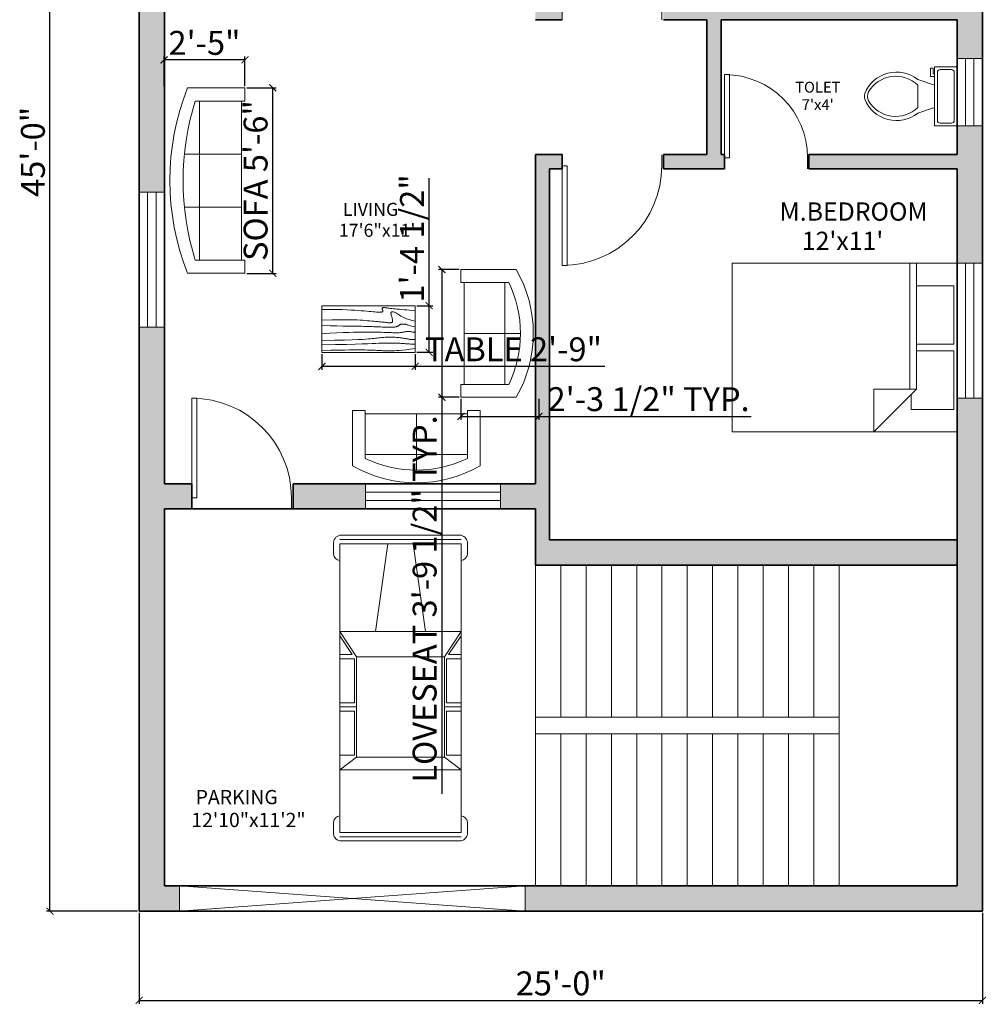
# Model space of a CAD drawing. Units: inches. Extents: x 3799 to 20199, y 1682 to 8087.
# Tile 26 of 30: x 16248 to 16592, y 7462 to 7812. Entities that reach past the tile are written whole.
import ezdxf

# ---------------------------------------------------------------- set-up
doc = ezdxf.new("R2010")
doc.units = ezdxf.units.IN
for name, color, linetype, lineweight in [('A-ANNO-DIMS', 2, 'Continuous', 18), ('A-AREA-IDEN', 7, 'Continuous', 18), ('A-DOOR', 3, 'Continuous', 18), ('A-FLOR-FIXT', 9, 'Continuous', 18), ('A-FLOR-STRS', 41, 'Continuous', 18), ('A-FURN', 8, 'Continuous', 18), ('A-GLAZ', 152, 'Continuous', 18), ('A-SITE-VEHC', 8, 'Continuous', 13), ('A-WALL', 7, 'Continuous', 35), ('A-WALL-PATT', 252, 'Continuous', 13)]:
    doc.layers.add(name, color=color, linetype=linetype, lineweight=lineweight)
doc.styles.get("Standard").update_dxf_attribs({"font": 'arial.ttf'})
doc.dimstyles.new('ISO-25', dxfattribs={"dimtxt": 8.5, "dimasz": 2.5, "dimexe": 1.25, "dimexo": 0.625, "dimtad": 1, "dimdec": 0, "dimlunit": 3, "dimtxsty": 'Standard', "dimblk": 'ARCHTICK', "dimcen": 2.5, "dimadec": 0, "dimazin": 0, "dimtfac": 1, "dimtdec": 0, "dimtmove": 0, "dimatfit": 3, "dimfxl": 1, "dimarcsym": 0})

# ---------------------------------------------------------------- blocks, each defined once
blk = doc.blocks.new('Sofa - Roundback Loveseat 5 ft.')
for p, q in [((0, -32.44198), (0, -5.99998)), ((-24, -33.99998), (-24, -11.46958)), ((-23.9998, -13.38178), (23.99986, -13.38178)), ((24.00004, -33.99998), (24.00004, -11.46958)), ((-24, -32.44198), (24.00004, -32.44198))]:
    blk.add_line(p, q)
for points in [[(-24, -33.99998), (-30, -33.99998), (-30, -7.99998)], [(30.00004, -7.99998), (30.00004, -33.99998), (24.00004, -33.99998)]]:
    blk.add_lwpolyline(points)
for centre, radius, start, end in [((0, -60.24998), 60.24998, 60.13715, 119.8628), ((0, -61.38438), 55.38444, 64.32083, 115.6792)]:
    blk.add_arc(centre, radius, start, end)
blk = doc.blocks.new('Sofa - Roundback 7 ft.')
for p, q in [((-12.00002, -32.4421), (-12.00003, -6.5971)), ((11.99997, -32.4421), (11.99998, -6.5971)), ((-36.000027, -34), (-36.000027, -11.4696)), ((35.99998, -34), (35.99998, -11.4696)), ((-35.999844, -13.3819), (35.9998, -13.3819)), ((-36.000027, -32.4421), (35.99998, -32.4421))]:
    blk.add_line(p, q)
for points in [[(-36.000027, -34), (-42.000027, -34), (-42.000027, -8)], [(41.99998, -8), (41.99998, -34), (35.99998, -34)]]:
    blk.add_lwpolyline(points)
for centre, radius, start, end in [((0, -114.25), 114.25, 68.43141, 111.5686), ((-0.00001, -127.1968), 121.1968, 72.72033, 107.2797)]:
    blk.add_arc(centre, radius, start, end)
blk = doc.blocks.new('Table - Rectangular Woodgrain 60 x 30 in.')
for p, q in [((0, 0), (0, -30)), ((60, 0), (0, 0)), ((60, -30), (60, 0)), ((0, -30), (60, -30))]:
    blk.add_line(p, q)
for points in [[(0, -2.4), (4.8155, -2.418), (9.0302, -2.4688), (12.709, -2.5477), (15.9167, -2.65), (18.7181, -2.7711), (21.1781, -2.9063), (23.3616, -3.0508), (25.3333, -3.2), (27.1477, -3.3495), (28.8172, -3.4958), (30.3437, -3.636), (31.7291, -3.7667), (32.9756, -3.8849), (34.0849, -3.9875), (35.059, -4.0714), (35.9, -4.1334), (36.6114, -4.1711), (37.2041, -4.1854), (37.6906, -4.1779), (38.0833, -4.15), (38.3948, -4.1034), (38.6375, -4.0396), (38.8239, -3.9602), (38.9666, -3.8667), (39.0764, -3.7608), (39.1573, -3.6448), (39.2116, -3.521), (39.2416, -3.3917), (39.2498, -3.2593), (39.2385, -3.1261), (39.21, -2.9944), (39.1666, -2.8667), (39.111, -2.7447), (39.0468, -2.6281), (38.978, -2.5163), (38.9083, -2.4083), (38.8418, -2.3035), (38.7823, -2.201), (38.7337, -2.1001), (38.7, -2), (38.6844, -1.9003), (38.6875, -1.8021), (38.7094, -1.707), (38.75, -1.6167), (38.8094, -1.5326), (38.8875, -1.4563), (38.9844, -1.3893), (39.1, -1.3333), (39.2351, -1.2896), (39.3937, -1.2583), (39.5804, -1.2396), (39.8, -1.2333), (40.057, -1.2396), (40.3562, -1.2583), (40.7023, -1.2896), (41.1, -1.3333), (41.5547, -1.3895), (42.0755, -1.4573), (42.6721, -1.5361), (43.3542, -1.625), (44.1316, -1.7233), (45.014, -1.8302), (46.0114, -1.9449), (47.1333, -2.0667), (48.3862, -2.1947), (49.7625, -2.3281), (51.2513, -2.4663), (52.8416, -2.6083), (54.5226, -2.7535), (56.2833, -2.9011), (58.1127, -3.0501), (60, -3.2)], [(0, -9.2), (6.5759, -9.0858), (11.9385, -9.0365), (16.2527, -9.0418), (19.6833, -9.0917), (22.3952, -9.1759), (24.5531, -9.2844), (26.322, -9.4069), (27.8666, -9.5333), (29.3241, -9.6553), (30.7203, -9.7719), (32.0532, -9.8837), (33.3208, -9.9917), (34.5213, -10.0965), (35.6526, -10.199), (36.7128, -10.2999), (37.7, -10.4), (38.6129, -10.4996), (39.4531, -10.5969), (40.223, -10.6895), (40.925, -10.775), (41.5613, -10.8512), (42.1344, -10.9156), (42.6465, -10.966), (43.1, -11), (43.4976, -11.0158), (43.8437, -11.0136), (44.143, -10.9942), (44.4, -10.9583), (44.6195, -10.9069), (44.8062, -10.8406), (44.9648, -10.7603), (45.1, -10.6667), (45.2155, -10.5598), (45.3114, -10.4365), (45.3871, -10.2929), (45.4416, -10.125), (45.4743, -9.929), (45.4844, -9.7011), (45.4709, -9.4371), (45.4333, -9.1333), (45.3716, -8.7883), (45.2896, -8.4104), (45.1919, -8.0107), (45.0833, -7.6), (44.9685, -7.1893), (44.8521, -6.7896), (44.7388, -6.4117), (44.6333, -6.0667), (44.54, -5.7628), (44.4614, -5.4979), (44.4001, -5.2675), (44.3583, -5.0667), (44.3384, -4.8909), (44.3427, -4.7354), (44.3736, -4.5956), (44.4333, -4.4667), (44.5236, -4.3453), (44.6427, -4.2333), (44.7884, -4.1339), (44.9583, -4.05), (45.1501, -3.9849), (45.3614, -3.9417), (45.59, -3.9234), (45.8333, -3.9333), (46.0915, -3.9749), (46.3734, -4.0531), (46.6906, -4.1736), (47.0542, -4.3417), (47.4756, -4.5629), (47.9661, -4.8427), (48.5372, -5.1866), (49.2, -5.6), (49.9676, -6.0844), (50.8594, -6.625), (51.8965, -7.2031), (53.1, -7.8), (54.491, -8.3969), (56.0906, -8.975), (57.9199, -9.5156), (60, -10)], [(0, -12.8), (5.1847, -12.9322), (9.6213, -13.0323), (13.3963, -13.1059), (16.5958, -13.1583), (19.3063, -13.1952), (21.614, -13.2219), (23.6054, -13.2439), (25.3666, -13.2667), (26.9728, -13.2947), (28.4531, -13.3281), (29.8256, -13.3663), (31.1083, -13.4083), (32.3191, -13.4535), (33.476, -13.501), (34.597, -13.5501), (35.7, -13.6), (36.7984, -13.6497), (37.8875, -13.6979), (38.9578, -13.743), (40, -13.7833), (41.0047, -13.8174), (41.9625, -13.8438), (42.864, -13.8607), (43.7, -13.8667), (44.4631, -13.8604), (45.1552, -13.8417), (45.7801, -13.8104), (46.3416, -13.7667), (46.8439, -13.7104), (47.2906, -13.6417), (47.6858, -13.5604), (48.0333, -13.4667), (48.3375, -13.3608), (48.6042, -13.2448), (48.8396, -13.121), (49.05, -12.9917), (49.2417, -12.8593), (49.4208, -12.7261), (49.5937, -12.5944), (49.7667, -12.4667), (49.9452, -12.3451), (50.1323, -12.2313), (50.3303, -12.1268), (50.5416, -12.0333), (50.7686, -11.9524), (51.0135, -11.8854), (51.2788, -11.8341), (51.5666, -11.8), (51.8785, -11.7843), (52.2116, -11.7865), (52.562, -11.8059), (52.926, -11.8417), (53.2998, -11.8931), (53.6795, -11.9594), (54.0614, -12.0397), (54.4416, -12.1333), (54.8223, -12.2401), (55.2293, -12.3625), (55.6942, -12.5037), (56.2489, -12.6667), (56.9251, -12.8547), (57.7545, -13.0708), (58.7689, -13.3182), (60, -13.6)], [(0, -18), (5.124, -17.7273), (9.6609, -17.5057), (13.6705, -17.3303), (17.2125, -17.1958), (20.3467, -17.0973), (23.1328, -17.0297), (25.6307, -16.9878), (27.9, -16.9667), (29.9928, -16.9617), (31.9302, -16.9703), (33.7254, -16.9907), (35.3917, -17.0208), (36.9423, -17.0588), (38.3906, -17.1026), (39.7499, -17.1503), (41.0333, -17.2), (42.2519, -17.2496), (43.4073, -17.2969), (44.4986, -17.3395), (45.525, -17.375), (46.4858, -17.4012), (47.3802, -17.4156), (48.2074, -17.416), (48.9667, -17.4), (49.6583, -17.3662), (50.2872, -17.3167), (50.8595, -17.2547), (51.3812, -17.1833), (51.8584, -17.1057), (52.2971, -17.025), (52.7034, -16.9443), (53.0833, -16.8667), (53.443, -16.7951), (53.789, -16.7313), (54.128, -16.6768), (54.4666, -16.6334), (54.8115, -16.6024), (55.1693, -16.5854), (55.5465, -16.5841), (55.95, -16.6), (56.3828, -16.6337), (56.8346, -16.6823), (57.2915, -16.7418), (57.7396, -16.8084), (58.165, -16.878), (58.5539, -16.9469), (58.8924, -17.0111), (59.1666, -17.0667), (59.3679, -17.1107), (59.5078, -17.1438), (59.6032, -17.1675), (59.6708, -17.1833), (59.7275, -17.193), (59.7901, -17.1979), (59.8753, -17.1998), (60, -17.2)], [(0, -22.4), (8.0098, -22.2501), (14.4094, -22.1011), (19.4168, -21.9535), (23.25, -21.8083), (26.1269, -21.6663), (28.2656, -21.5281), (29.884, -21.3947), (31.2, -21.2667), (32.3967, -21.1448), (33.5172, -21.0292), (34.5697, -20.9198), (35.5625, -20.8167), (36.5037, -20.7198), (37.4015, -20.6292), (38.2642, -20.5448), (39.1, -20.4667), (39.9164, -20.3951), (40.7187, -20.3313), (41.5117, -20.2768), (42.3, -20.2333), (43.0883, -20.2024), (43.8812, -20.1854), (44.6836, -20.1841), (45.5, -20.2), (46.3328, -20.234), (47.1747, -20.2844), (48.0163, -20.3488), (48.8479, -20.425), (49.66, -20.5106), (50.4429, -20.6031), (51.1872, -20.7004), (51.8833, -20.8), (52.5246, -20.8999), (53.1166, -20.9995), (53.6681, -21.0983), (54.1875, -21.1958), (54.6834, -21.2919), (55.1646, -21.3859), (55.6394, -21.4777), (56.1167, -21.5667), (56.6028, -21.6515), (57.0961, -21.7266), (57.5929, -21.7852), (58.0896, -21.8208), (58.5823, -21.8268), (59.0674, -21.7964), (59.5412, -21.723), (60, -21.6)], [(0, -25.2), (8.6355, -25.0504), (15.7026, -24.9031), (21.4049, -24.7606), (25.9458, -24.625), (29.529, -24.4988), (32.3578, -24.3844), (34.6359, -24.284), (36.5667, -24.2), (38.3213, -24.1341), (39.9417, -24.0854), (41.437, -24.0523), (42.8167, -24.0333), (44.0901, -24.0268), (45.2667, -24.0313), (46.3557, -24.0451), (47.3667, -24.0667), (48.309, -24.0947), (49.1928, -24.1287), (50.0284, -24.168), (50.826, -24.2125), (51.5959, -24.2617), (52.3483, -24.3151), (53.0935, -24.3725), (53.8417, -24.4334), (54.6009, -24.497), (55.3699, -24.561), (56.1454, -24.6226), (56.9239, -24.6792), (57.7021, -24.7279), (58.4764, -24.7662), (59.2435, -24.7911), (60, -24.8)], [(0, -28.8), (5.6867, -28.6681), (10.45, -28.5698), (14.407, -28.5012), (17.675, -28.4584), (20.3711, -28.4374), (22.6125, -28.4344), (24.5164, -28.4455), (26.2, -28.4667), (27.762, -28.4947), (29.2276, -28.5281), (30.6033, -28.5663), (31.8958, -28.6084), (33.1118, -28.6535), (34.2578, -28.7011), (35.3405, -28.7501), (36.3666, -28.8), (37.3443, -28.8497), (38.288, -28.8974), (39.2137, -28.9412), (40.1375, -28.9792), (41.0753, -29.0093), (42.0432, -29.0297), (43.0572, -29.0384), (44.1333, -29.0333), (45.2936, -29.0114), (46.5843, -28.9641), (48.0579, -28.8816), (49.7666, -28.7542), (51.7629, -28.5721), (54.0989, -28.3255), (56.8272, -28.0048), (60, -27.6)]]:
    blk.add_lwpolyline(points)
blk = doc.blocks.new('*U157')
for p, q in [((0.1, -0.41), (0.1, 38.35)), ((2.77, -0.41), (2.77, 38.31)), ((5.44, 42.31), (12.12, 42.31)), ((5.44, -0.41), (5.44, 38.24)), ((5.45, 38.31), (16.12, 38.31)), ((16.12, 38.31), (180.34, 38.31)), ((61.52, -0.41), (61.52, 38.31)), ((61.52, 38.31), (77.54, 27.62)), ((64.19, 38.31), (76.2, 30.29)), ((76.2, 30.29), (76.2, 38.31)), ((78.87, 38.31), (78.87, 28.96)), ((106.91, 28.96), (106.91, 38.31)), ((109.58, 27.62), (109.58, 38.31)), ((112.25, 38.31), (112.25, 28.96)), ((140.29, 28.96), (140.29, 38.31)), ((141.62, 27.62), (149.64, 38.31)), ((149.64, -0.41), (149.64, 38.31)), ((189.69, 38.31), (179.01, 38.31)), ((189.69, 42.31), (183.01, 42.31)), ((189.69, -0.41), (189.69, 38.24)), ((192.36, -0.41), (192.36, 38.31)), ((195.03, -0.41), (195.03, 38.35)), ((77.54, 27.62), (141.62, 27.62)), ((77.54, -0.41), (77.54, 27.62)), ((78.87, 28.96), (106.91, 28.96)), ((112.25, 28.96), (140.29, 28.96)), ((141.62, -0.41), (141.62, 27.62)), ((5.44, 7.6), (61.52, 15.61)), ((0.1, -0.42), (0.1, -39.18)), ((2.77, -0.41), (2.77, -39.13)), ((5.44, -0.42), (5.44, -39.07)), ((61.52, -0.41), (61.52, -39.13)), ((77.54, -0.41), (77.54, -28.45)), ((141.62, -0.41), (141.62, -28.45)), ((149.64, -0.41), (149.64, -39.13)), ((189.69, -0.42), (189.69, -39.07)), ((192.36, -0.41), (192.36, -39.13)), ((195.03, -0.42), (195.03, -39.18)), ((5.44, -8.42), (61.52, -16.43)), ((61.52, -39.13), (77.54, -28.45)), ((64.19, -39.13), (76.2, -31.12)), ((76.2, -31.12), (76.2, -39.13)), ((77.54, -28.45), (141.62, -28.45)), ((78.87, -39.13), (78.87, -29.79)), ((78.87, -29.79), (106.91, -29.79)), ((106.91, -29.79), (106.91, -39.13)), ((109.58, -28.45), (109.58, -39.13)), ((112.25, -29.79), (140.29, -29.79)), ((112.25, -39.13), (112.25, -29.79)), ((140.29, -29.79), (140.29, -39.13)), ((141.62, -28.45), (149.64, -39.13)), ((5.44, -43.14), (12.12, -43.14)), ((5.45, -39.13), (16.12, -39.13)), ((16.12, -39.13), (180.34, -39.13)), ((189.69, -39.13), (179.01, -39.13)), ((189.69, -43.14), (183.01, -43.14))]:
    blk.add_line(p, q)
for centre, radius, start, end in [((5.06, 37.26), 5.06, 85.64554, 168.0943), ((11.45, 37.64), 4.72, 8.13011, 81.86996), ((183.68, 37.64), 4.72, 98.13004, 171.8699), ((190.07, 37.26), 5.06, 11.90574, 94.35446), ((5.06, -38.09), 5.06, 191.9057, 274.3545), ((11.45, -38.46), 4.72, 278.13, 351.8699), ((183.68, -38.46), 4.72, 188.1301, 261.87), ((190.07, -38.09), 5.06, 265.6455, 348.0943)]:
    blk.add_arc(centre, radius, start, end)
blk = doc.blocks.new('*U49')
for p, q in [((0, 0), (0, -100)), ((900, 0), (900, -100))]:
    blk.add_line(p, q)
blk.add_lwpolyline([(0, 0), (0, 900), (43.75, 900), (43.75, 0)], close=True)
blk.add_arc((0, 0), 900, 0, 90)
blk = doc.blocks.new('*U47')
for p, q in [((0, 0), (0, -100)), ((750, 0), (750, -100))]:
    blk.add_line(p, q)
blk.add_lwpolyline([(0, 0), (0, 750), (43.75, 750), (43.75, 0)], close=True)
blk.add_arc((0, 0), 750, 0, 90)
blk = doc.blocks.new('*U156')
for p, q in [((0, 0), (0, 100)), ((900, 0), (900, 100))]:
    blk.add_line(p, q)
blk.add_lwpolyline([(0, 0), (0, -900), (43.75, -900), (43.75, 0)], close=True)
blk.add_arc((0, 0), 900, 270, 0)
blk = doc.blocks.new('Bed - Queen')
for p, q in [((0, -80.00003), (0, 0)), ((0, 0), (59.99999, 0)), ((59.99999, 0), (59.99999, -80.00003)), ((7.99999, -1.2), (28.79998, -1.2)), ((7.99999, -14.4), (7.99999, -1.2)), ((28.79998, -1.2), (28.79998, -14.4)), ((31.19999, -1.2), (51.99999, -1.2)), ((31.19999, -14.4), (31.19999, -1.2)), ((51.99999, -1.2), (51.99999, -16.4)), ((0, -14.4), (44.8, -14.4)), ((44.8, -16.8), (0, -16.8)), ((59.99999, -29.6), (44.8, -14.4)), ((44.8, -14.4), (44.8, -29.6)), ((51.99999, -16.4), (46.79936, -16.4)), ((44.8, -29.6), (59.99999, -29.6)), ((59.99999, -80.00003), (0, -80.00003))]:
    blk.add_line(p, q)
blk = doc.blocks.new('Toilet - top')
for p, q in [((9.5, -6), (9.5, -2)), ((-10, -8.5), (-8, -8.5)), ((-10, -9.5), (-10, -8.5)), ((-7, -9.5), (-10, -9.5)), ((-8, -8.5), (-8, -8)), ((-7, -8), (-7, -9.5)), ((-4, -8), (-6, -14)), ((4, -8), (6, -14)), ((4, -14), (-4, -14))]:
    blk.add_line(p, q)
blk.add_lwpolyline([(10.5, -8), (10.5, 0), (-10.5, 0), (-10.5, -8)], close=True)
for points in [[(-9.5, -2), (-9.5, -6)], [(8.5, -1), (-8.5, -1)], [(-8.5, -7), (8.5, -7)]]:
    blk.add_lwpolyline(points)
for centre, radius, start, end in [((-8.62, -1.88), 0.884, 81.8699, 188.1301), ((8.62, -1.88), 0.884, 351.8699, 98.1301), ((-8.62, -6.12), 0.884, 171.8699, 278.1301), ((8.62, -6.12), 0.884, 261.8699, 8.1301), ((3.52, -21.58), 12.17, 141.4691, 247.9714), ((4.2, -21.82), 11.33, 136.3677, 238.9468), ((-3.52, -21.58), 12.17, 292.0284, 38.5307), ((-4.2, -21.82), 11.33, 301.053, 43.6321), ((0, -27.88), 4, 245.7318, 294.2682), ((0, -29), 4, 254.8605, 285.1395)]:
    blk.add_arc(centre, radius, start, end)
blk = doc.blocks.new('WIN-24IN-9IN-FRAME')
for p, q in [((0, 24), (9, 24)), ((3, 0), (3, 24)), ((6, 0), (6, 24)), ((0, 0), (9, 0))]:
    blk.add_line(p, q)
blk = doc.blocks.new('WIN-48IN-9IN-FRAME')
for p, q in [((0, 0), (0, 9)), ((48, 0), (48, 9)), ((48, 6), (0, 6)), ((48, 3), (0, 3))]:
    blk.add_line(p, q)
blk = doc.blocks.new('_ArchTick')
at = {"color": 0, "linetype": 'ByBlock', "const_width": 0.15}
blk.add_lwpolyline([(-0.5, -0.5), (0.5, 0.5)], dxfattribs=at)
blk = doc.blocks.new('*D262')
at = {"layer": 'A-ANNO-DIMS', "color": 0, "lineweight": -2, "transparency": 16777216}
for p, q in [((16328.6, 7787.44), (16339.12, 7787.44)), ((16337.87, 7721.45), (16337.87, 7787.44)), ((16328.6, 7721.45), (16339.12, 7721.45))]:
    blk.add_line(p, q, dxfattribs=at)
at = {"layer": 'Defpoints', "color": 0, "transparency": 16777216}
for p in [(16327.97, 7787.44), (16337.87, 7787.44), (16327.97, 7721.45)]:
    blk.add_point(p, dxfattribs=at)
at = {"layer": 'A-ANNO-DIMS', "color": 0, "lineweight": -2, "transparency": 16777216, "xscale": 2.5, "yscale": 2.5, "zscale": 2.5}
for p, rotation in [((16337.87, 7787.44), 90), ((16337.87, 7721.45), 270)]:
    blk.add_blockref('_ArchTick', p, dxfattribs=dict(at, rotation=rotation))
at = {"layer": 'A-ANNO-DIMS', "color": 0, "transparency": 16777216, "insert": (16332.85, 7754.45), "char_height": 8.5, "attachment_point": 5, "rotation": 90}
blk.add_mtext('SOFA 5\'-6"', dxfattribs=at)
blk = doc.blocks.new('*D263')
at = {"layer": 'A-ANNO-DIMS', "color": 0, "lineweight": -2, "transparency": 16777216}
for p, q in [((16299.17, 7788.06), (16299.17, 7798.59)), ((16327.97, 7788.06), (16327.97, 7798.59)), ((16327.97, 7797.34), (16299.17, 7797.34))]:
    blk.add_line(p, q, dxfattribs=at)
at = {"layer": 'Defpoints', "color": 0, "transparency": 16777216}
for p in [(16299.17, 7797.34), (16299.17, 7787.44), (16327.97, 7787.44)]:
    blk.add_point(p, dxfattribs=at)
at = {"layer": 'A-ANNO-DIMS', "color": 0, "lineweight": -2, "transparency": 16777216, "xscale": 2.5, "yscale": 2.5, "zscale": 2.5, "rotation": 180}
blk.add_blockref('_ArchTick', (16299.17, 7797.34), dxfattribs=at)
at = {"layer": 'A-ANNO-DIMS', "color": 0, "lineweight": -2, "transparency": 16777216, "xscale": 2.5, "yscale": 2.5, "zscale": 2.5}
blk.add_blockref('_ArchTick', (16327.97, 7797.34), dxfattribs=at)
at = {"layer": 'A-ANNO-DIMS', "color": 0, "transparency": 16777216, "insert": (16313.57, 7802.3), "char_height": 8.5, "attachment_point": 5}
blk.add_mtext('2\'-5"', dxfattribs=at)
blk = doc.blocks.new('*D278')
at = {"layer": 'A-ANNO-DIMS', "color": 0, "lineweight": -2, "transparency": 16777216}
for p, q in [((16404.2, 7722.78), (16396.77, 7722.78)), ((16398.02, 7722.78), (16398.02, 7677.4)), ((16404.2, 7677.4), (16396.77, 7677.4)), ((16398.02, 7677.4), (16398.02, 7536.41))]:
    blk.add_line(p, q, dxfattribs=at)
at = {"layer": 'Defpoints', "color": 0, "transparency": 16777216}
for p in [(16404.82, 7722.78), (16398.02, 7677.4), (16404.82, 7677.4)]:
    blk.add_point(p, dxfattribs=at)
at = {"layer": 'A-ANNO-DIMS', "color": 0, "lineweight": -2, "transparency": 16777216, "xscale": 2.5, "yscale": 2.5, "zscale": 2.5}
for p, rotation in [((16398.02, 7722.78), 90), ((16398.02, 7677.4), 270)]:
    blk.add_blockref('_ArchTick', p, dxfattribs=dict(at, rotation=rotation))
at = {"layer": 'A-ANNO-DIMS', "color": 0, "transparency": 16777216, "insert": (16392.99, 7605.65), "char_height": 8.5, "attachment_point": 5, "rotation": 90}
blk.add_mtext('LOVESEAT 3\'-9 1/2" TYP.', dxfattribs=at)
blk = doc.blocks.new('*D279')
at = {"layer": 'A-ANNO-DIMS', "color": 0, "lineweight": -2, "transparency": 16777216}
for p, q in [((16404.82, 7676.77), (16404.82, 7669.34)), ((16432.56, 7676.77), (16432.56, 7669.34)), ((16404.82, 7670.59), (16432.56, 7670.59)), ((16432.56, 7670.59), (16508.07, 7670.59))]:
    blk.add_line(p, q, dxfattribs=at)
at = {"layer": 'Defpoints', "color": 0, "transparency": 16777216}
for p in [(16404.82, 7677.4), (16432.56, 7677.4), (16432.56, 7670.59)]:
    blk.add_point(p, dxfattribs=at)
at = {"layer": 'A-ANNO-DIMS', "color": 0, "lineweight": -2, "transparency": 16777216, "xscale": 2.5, "yscale": 2.5, "zscale": 2.5, "rotation": 180}
blk.add_blockref('_ArchTick', (16404.82, 7670.59), dxfattribs=at)
at = {"layer": 'A-ANNO-DIMS', "color": 0, "lineweight": -2, "transparency": 16777216, "xscale": 2.5, "yscale": 2.5, "zscale": 2.5}
blk.add_blockref('_ArchTick', (16432.56, 7670.59), dxfattribs=at)
at = {"layer": 'A-ANNO-DIMS', "color": 0, "transparency": 16777216, "insert": (16471.57, 7675.61), "char_height": 8.5, "attachment_point": 5}
blk.add_mtext('2\'-3 1/2" TYP.', dxfattribs=at)
blk = doc.blocks.new('*D332')
at = {"layer": 'A-ANNO-DIMS', "color": 0, "lineweight": -2, "transparency": 16777216}
for p, q in [((16355.36, 7692.73), (16355.36, 7687.13)), ((16388.53, 7692.73), (16388.53, 7687.13)), ((16355.36, 7688.38), (16388.53, 7688.38)), ((16388.53, 7688.38), (16456.01, 7688.38))]:
    blk.add_line(p, q, dxfattribs=at)
at = {"layer": 'Defpoints', "color": 0, "transparency": 16777216}
for p in [(16355.36, 7693.36), (16388.53, 7693.36), (16388.53, 7688.38)]:
    blk.add_point(p, dxfattribs=at)
at = {"layer": 'A-ANNO-DIMS', "color": 0, "lineweight": -2, "transparency": 16777216, "xscale": 2.5, "yscale": 2.5, "zscale": 2.5, "rotation": 180}
blk.add_blockref('_ArchTick', (16355.36, 7688.38), dxfattribs=at)
at = {"layer": 'A-ANNO-DIMS', "color": 0, "lineweight": -2, "transparency": 16777216, "xscale": 2.5, "yscale": 2.5, "zscale": 2.5}
blk.add_blockref('_ArchTick', (16388.53, 7688.38), dxfattribs=at)
at = {"layer": 'A-ANNO-DIMS', "color": 0, "transparency": 16777216, "insert": (16423.52, 7693.35), "char_height": 8.5, "attachment_point": 5}
blk.add_mtext('TABLE 2\'-9"', dxfattribs=at)
blk = doc.blocks.new('*D333')
at = {"layer": 'A-ANNO-DIMS', "color": 0, "lineweight": -2, "transparency": 16777216}
for p, q in [((16393.51, 7709.94), (16393.51, 7755.29)), ((16389.16, 7709.94), (16394.76, 7709.94)), ((16393.51, 7693.36), (16393.51, 7709.94)), ((16389.16, 7693.36), (16394.76, 7693.36))]:
    blk.add_line(p, q, dxfattribs=at)
at = {"layer": 'Defpoints', "color": 0, "transparency": 16777216}
for p in [(16388.53, 7709.94), (16393.51, 7709.94), (16388.53, 7693.36)]:
    blk.add_point(p, dxfattribs=at)
at = {"layer": 'A-ANNO-DIMS', "color": 0, "lineweight": -2, "transparency": 16777216, "xscale": 2.5, "yscale": 2.5, "zscale": 2.5}
for p, rotation in [((16393.51, 7709.94), 90), ((16393.51, 7693.36), 270)]:
    blk.add_blockref('_ArchTick', p, dxfattribs=dict(at, rotation=rotation))
at = {"layer": 'A-ANNO-DIMS', "color": 0, "transparency": 16777216, "insert": (16388.49, 7733.87), "char_height": 8.5, "attachment_point": 5, "rotation": 90}
blk.add_mtext('1\'-4 1/2"', dxfattribs=at)
blk = doc.blocks.new('*D358')
at = {"layer": 'A-ANNO-DIMS', "color": 0, "lineweight": -2, "transparency": 16777216}
for p, q in [((16290.33, 7494.02), (16290.33, 7461.65)), ((16590.33, 7494.02), (16590.33, 7461.65)), ((16290.33, 7462.9), (16590.33, 7462.9))]:
    blk.add_line(p, q, dxfattribs=at)
at = {"layer": 'Defpoints', "color": 0, "transparency": 16777216}
for p in [(16290.33, 7494.65), (16590.33, 7494.65), (16590.33, 7462.9)]:
    blk.add_point(p, dxfattribs=at)
at = {"layer": 'A-ANNO-DIMS', "color": 0, "lineweight": -2, "transparency": 16777216, "xscale": 2.5, "yscale": 2.5, "zscale": 2.5, "rotation": 180}
blk.add_blockref('_ArchTick', (16290.33, 7462.9), dxfattribs=at)
at = {"layer": 'A-ANNO-DIMS', "color": 0, "lineweight": -2, "transparency": 16777216, "xscale": 2.5, "yscale": 2.5, "zscale": 2.5}
blk.add_blockref('_ArchTick', (16590.33, 7462.9), dxfattribs=at)
at = {"layer": 'A-ANNO-DIMS', "color": 0, "transparency": 16777216, "insert": (16440.33, 7467.86), "char_height": 8.5, "attachment_point": 5}
blk.add_mtext('25\'-0"', dxfattribs=at)
blk = doc.blocks.new('*D359')
at = {"layer": 'A-ANNO-DIMS', "color": 0, "lineweight": -2, "transparency": 16777216}
for p, q in [((16289.71, 8034.65), (16257.33, 8034.65)), ((16258.58, 7494.65), (16258.58, 8034.65)), ((16289.71, 7494.65), (16257.33, 7494.65))]:
    blk.add_line(p, q, dxfattribs=at)
at = {"layer": 'Defpoints', "color": 0, "transparency": 16777216}
for p in [(16258.58, 8034.65), (16290.33, 8034.65), (16290.33, 7494.65)]:
    blk.add_point(p, dxfattribs=at)
at = {"layer": 'A-ANNO-DIMS', "color": 0, "lineweight": -2, "transparency": 16777216, "xscale": 2.5, "yscale": 2.5, "zscale": 2.5}
for p, rotation in [((16258.58, 8034.65), 90), ((16258.58, 7494.65), 270)]:
    blk.add_blockref('_ArchTick', p, dxfattribs=dict(at, rotation=rotation))
at = {"layer": 'A-ANNO-DIMS', "color": 0, "transparency": 16777216, "insert": (16253.62, 7764.65), "char_height": 8.5, "attachment_point": 5, "rotation": 90}
blk.add_mtext('45\'-0"', dxfattribs=at)

msp = doc.modelspace()

# ---------------------------------------------------------------- hatches: boundary and pattern name
at = {"layer": 'A-WALL-PATT'}
h = msp.add_hatch(color=256, dxfattribs=at)
h.dxf.hatch_style = 1
h.paths.add_polyline_path([(16358.47, 8034.65), (16290.33, 8034.65), (16290.33, 8012.2), (16294.27, 8012.2), (16299.33, 8012.2), (16299.33, 8025.65), (16358.47, 8025.65)])
h.paths.add_polyline_path([(16463.1, 8034.65), (16406.47, 8034.65), (16406.47, 8025.65), (16431.33, 8025.65), (16431.33, 7994.23), (16436.33, 7994.23), (16436.33, 8025.65), (16463.1, 8025.65)])
h.paths.add_polyline_path([(16549.72, 8034.65), (16511.1, 8034.65), (16511.1, 8025.65), (16528.33, 8025.65), (16528.33, 7941.65), (16436.33, 7941.65), (16436.33, 7946.23), (16431.33, 7946.23), (16431.33, 7905.65), (16422.55, 7905.65), (16422.55, 7896.65), (16431.33, 7896.65), (16431.33, 7811.65), (16440.82, 7811.65), (16440.82, 7816.65), (16436.33, 7816.65), (16436.33, 7936.65), (16533.33, 7936.65), (16535.49, 7936.65), (16535.49, 7941.65), (16533.33, 7941.65), (16533.33, 8025.65), (16549.72, 8025.65)])
h.paths.add_polyline_path([(16590.33, 8034.65), (16573.72, 8034.65), (16573.72, 8025.65), (16581.33, 8025.65), (16581.33, 7941.65), (16565.49, 7941.65), (16565.49, 7936.65), (16581.33, 7936.65), (16581.33, 7908.97), (16590.33, 7908.97)])
h.paths.add_polyline_path([(16590.33, 7860.97), (16581.33, 7860.97), (16581.33, 7853.17), (16581.33, 7816.65), (16476.82, 7816.65), (16476.82, 7811.65), (16492.33, 7811.65), (16492.33, 7763.65), (16476.82, 7763.65), (16476.82, 7758.65), (16498.62, 7758.65), (16498.62, 7762.58), (16498.62, 7763.65), (16497.33, 7763.65), (16497.33, 7811.65), (16581.33, 7811.65), (16581.33, 7797.89), (16590.33, 7797.89)])
h.paths.add_polyline_path([(16590.33, 7773.89), (16581.33, 7773.89), (16581.33, 7763.65), (16528.62, 7763.65), (16528.62, 7758.65), (16581.33, 7758.65), (16581.33, 7725.04), (16590.33, 7725.04)])
h.paths.add_polyline_path([(16590.33, 7677.04), (16581.33, 7677.04), (16581.33, 7665.04), (16581.33, 7626.65), (16581.33, 7503.65), (16427.6, 7503.65), (16427.6, 7494.65), (16590.33, 7494.65)])
h.paths.add_polyline_path([(16581.33, 7626.65), (16436.33, 7626.65), (16436.33, 7758.65), (16440.82, 7758.65), (16440.82, 7759.71), (16440.82, 7763.65), (16431.33, 7763.65), (16431.33, 7646.65), (16418.83, 7646.65), (16418.83, 7637.65), (16431.33, 7637.65), (16431.33, 7617.65), (16581.33, 7617.65)])
h.paths.add_polyline_path([(16309.09, 7646.65), (16299.33, 7646.65), (16299.33, 7702.3), (16290.33, 7702.3), (16290.33, 7494.65), (16304.67, 7494.65), (16304.67, 7503.65), (16299.33, 7503.65), (16299.33, 7637.65), (16309.09, 7637.65), (16309.09, 7641.58)])
h.paths.add_polyline_path([(16299.33, 7896.65), (16374.55, 7896.65), (16374.55, 7905.65), (16299.33, 7905.65), (16299.33, 7976.2), (16290.33, 7976.2), (16290.33, 7750.3), (16299.33, 7750.3)])
h.paths.add_polyline_path([(16370.83, 7646.65), (16345.09, 7646.65), (16345.09, 7637.65), (16370.83, 7637.65)])

# ---------------------------------------------------------------- linework, layer by layer
at = {"layer": 'A-DOOR'}
for p, q in [((16304.67, 7503.65), (16304.67, 7494.65)), ((16304.67, 7503.65), (16427.6, 7494.65)), ((16427.6, 7503.65), (16304.67, 7494.65)), ((16427.6, 7503.65), (16427.6, 7494.65))]:
    msp.add_line(p, q, dxfattribs=at)
at = {"layer": 'A-FLOR-STRS'}
for p, q in [((16431.33, 7617.65), (16431.33, 7503.65)), ((16440.33, 7617.65), (16440.33, 7563.65)), ((16449.33, 7617.65), (16449.33, 7563.65)), ((16458.33, 7617.65), (16458.33, 7563.65)), ((16467.33, 7617.65), (16467.33, 7563.65)), ((16476.33, 7617.65), (16476.33, 7563.65)), ((16485.33, 7617.65), (16485.33, 7563.65)), ((16494.33, 7617.65), (16494.33, 7563.65)), ((16503.33, 7617.65), (16503.33, 7563.65)), ((16512.33, 7617.65), (16512.33, 7563.65)), ((16521.33, 7617.65), (16521.33, 7563.65)), ((16530.33, 7617.65), (16530.33, 7563.65)), ((16539.33, 7617.65), (16539.33, 7503.65)), ((16539.33, 7563.65), (16431.33, 7563.65)), ((16539.33, 7557.65), (16431.33, 7557.65)), ((16440.33, 7557.65), (16440.33, 7503.65)), ((16449.33, 7557.65), (16449.33, 7503.65)), ((16458.33, 7557.65), (16458.33, 7503.65)), ((16467.33, 7557.65), (16467.33, 7503.65)), ((16476.33, 7557.65), (16476.33, 7503.65)), ((16485.33, 7557.65), (16485.33, 7503.65)), ((16494.33, 7557.65), (16494.33, 7503.65)), ((16503.33, 7557.65), (16503.33, 7503.65)), ((16512.33, 7557.65), (16512.33, 7503.65)), ((16521.33, 7557.65), (16521.33, 7503.65)), ((16530.33, 7557.65), (16530.33, 7503.65))]:
    msp.add_line(p, q, dxfattribs=at)
at = {"layer": 'A-WALL'}
for p, q in [((16590.33, 7494.65), (16590.33, 8034.65)), ((16290.33, 7976.2), (16290.33, 7494.65)), ((16299.33, 7896.65), (16299.33, 7646.65)), ((16440.82, 7811.65), (16431.33, 7811.65)), ((16492.33, 7811.65), (16476.82, 7811.65)), ((16492.33, 7763.65), (16492.33, 7811.65)), ((16581.33, 7811.65), (16497.33, 7811.65)), ((16497.33, 7763.65), (16497.33, 7811.65)), ((16581.33, 7763.65), (16581.33, 7811.65)), ((16431.33, 7763.65), (16431.33, 7646.65)), ((16440.82, 7763.65), (16431.33, 7763.65)), ((16440.82, 7758.65), (16440.82, 7763.65)), ((16476.82, 7758.65), (16476.82, 7763.65)), ((16492.33, 7763.65), (16476.82, 7763.65)), ((16498.62, 7763.65), (16497.33, 7763.65)), ((16498.62, 7763.65), (16498.62, 7758.65)), ((16581.33, 7763.65), (16528.62, 7763.65)), ((16528.62, 7763.65), (16528.62, 7758.65)), ((16436.33, 7758.65), (16436.33, 7626.65)), ((16440.82, 7758.65), (16436.33, 7758.65)), ((16498.62, 7758.65), (16476.82, 7758.65)), ((16581.33, 7758.65), (16528.62, 7758.65)), ((16581.33, 7626.65), (16581.33, 7758.65)), ((16299.33, 7646.65), (16309.09, 7646.65)), ((16309.09, 7646.65), (16309.09, 7637.65)), ((16345.09, 7646.65), (16345.09, 7637.65)), ((16345.09, 7646.65), (16431.33, 7646.65)), ((16299.33, 7637.65), (16309.09, 7637.65)), ((16299.33, 7637.65), (16299.33, 7503.65)), ((16345.09, 7637.65), (16309.09, 7637.65)), ((16345.09, 7637.65), (16431.33, 7637.65)), ((16431.33, 7637.65), (16431.33, 7617.65)), ((16581.33, 7626.65), (16436.33, 7626.65)), ((16581.33, 7626.65), (16581.33, 7503.65)), ((16581.33, 7617.65), (16431.33, 7617.65)), ((16299.33, 7503.65), (16581.33, 7503.65)), ((16290.33, 7494.65), (16590.33, 7494.65))]:
    msp.add_line(p, q, dxfattribs=at)

# ---------------------------------------------------------------- block references
at = {"layer": 'A-DOOR', "xscale": 0.0393700787401575, "yscale": 0.0393700787401575, "zscale": 0.0393700787401575}
for name, p in [('*U49', (16440.82, 7815.58)), ('*U47', (16498.62, 7762.58)), ('*U156', (16440.82, 7759.71)), ('*U49', (16309.09, 7641.58))]:
    msp.add_blockref(name, p, dxfattribs=at)
at = {"layer": 'A-FLOR-FIXT', "rotation": 270}
msp.add_blockref('Toilet - top', (16581.33, 7784.39), dxfattribs=at)
at = {"layer": 'A-FURN'}
for name, p, xscale, yscale, zscale, rotation in [('Sofa - Roundback 7 ft.', (16301.26, 7754.45), 0.7855546975016733, 0.7855546975016733, 0.7855546975016733, 90), ('Sofa - Roundback Loveseat 5 ft.', (16430.54, 7700.09), 0.756455551207799, 0.756455551207799, 0.756455551207799, 270), ('Sofa - Roundback Loveseat 5 ft.', (16388.94, 7646.94), 0.756455551207799, 0.756455551207799, 0.756455551207799, 180)]:
    msp.add_blockref(name, p, dxfattribs=dict(at, xscale=xscale, yscale=yscale, zscale=zscale, rotation=rotation))
at = {"layer": 'A-FURN', "rotation": 270}
msp.add_blockref('Bed - Queen', (16581.33, 7725.04), dxfattribs=at)
at = {"layer": 'A-FURN', "xscale": 0.5528191980204789, "yscale": 0.5528191980204789, "zscale": 0.5528191980204789}
msp.add_blockref('Table - Rectangular Woodgrain 60 x 30 in.', (16355.36, 7709.94), dxfattribs=at)
at = {"layer": 'A-GLAZ'}
for name, p in [('WIN-24IN-9IN-FRAME', (16581.33, 7773.89)), ('WIN-48IN-9IN-FRAME', (16370.83, 7637.65))]:
    msp.add_blockref(name, p, dxfattribs=at)
at = {"layer": 'A-GLAZ', "rotation": 90}
for p in [(16299.33, 7702.3), (16590.33, 7677.04)]:
    msp.add_blockref('WIN-48IN-9IN-FRAME', p, dxfattribs=at)
at = {"layer": 'A-SITE-VEHC', "xscale": 0.5575296130447742, "yscale": 0.5575296130447742, "zscale": 0.5575296130447742, "rotation": 270}
msp.add_blockref('*U157', (16383.52, 7628.34), dxfattribs=at)

# ---------------------------------------------------------------- texts
at = {"layer": 'A-AREA-IDEN'}
for s, height, p in [('TOLET', 3.856, (16523.7, 7785.71)), ("  7'x4'", 3.856, (16523.7, 7779.51)), (' LIVING', 4.638, (16361.38, 7741.88)), ('M.BEDROOM', 6.484, (16518.16, 7740.18)), ('17\'6"x11\'', 4.638, (16361.38, 7734.43)), ("    12'x11'", 6.4836, (16518.16, 7729.76)), (' PARKING', 5.064, (16308.88, 7532.67)), ('12\'10"x11\'2"', 5.0638, (16308.88, 7524.53))]:
    msp.add_text(s, height=height, rotation=0.0017, dxfattribs=at).set_placement(p)

# ---------------------------------------------------------------- dimensions: what is measured, and where the dimension line sits
at = {"layer": 'A-ANNO-DIMS'}
for base, p1, p2, angle, picture, middle in [((16258.58, 8034.65), (16290.33, 7494.65), (16290.33, 8034.65), 90, '*D359', (16253.62, 7764.65)), ((16299.17, 7797.34), (16327.97, 7787.44), (16299.17, 7787.44), 180, '*D263', (16313.57, 7802.3)), ((16393.51, 7709.94), (16388.53, 7693.36), (16388.53, 7709.94), 90, '*D333', (16388.49, 7733.87))]:
    dim = msp.add_linear_dim(base=base, p1=p1, p2=p2, angle=angle, dimstyle='ISO-25', override={"dimdec": 1, "dimlfac": 1, "dimrnd": 0, "dimzin": 1, "dimdsep": 46, "dimlunit": 4, "dimfrac": 2}, dxfattribs=at)
    dim.commit()
    dim.dimension.update_dxf_attribs({"geometry": picture, "text_midpoint": middle})
for base, p1, p2, angle, text, picture, middle in [((16337.87, 7787.44), (16327.97, 7721.45), (16327.97, 7787.44), 90, 'SOFA <>', '*D262', (16332.85, 7754.45)), ((16398.02, 7677.4), (16404.82, 7722.78), (16404.82, 7677.4), 270, 'LOVESEAT <> TYP.', '*D278', (16392.99, 7605.65))]:
    dim = msp.add_linear_dim(base=base, p1=p1, p2=p2, angle=angle, text=text, dimstyle='ISO-25', override={"dimdec": 1, "dimlfac": 1, "dimrnd": 0, "dimzin": 1, "dimdsep": 46, "dimlunit": 4, "dimfrac": 2}, dxfattribs=at)
    dim.commit()
    dim.dimension.update_dxf_attribs({"geometry": picture, "text_midpoint": middle})
for base, p1, p2, text, picture, middle in [((16388.53, 7688.38), (16355.36, 7693.36), (16388.53, 7693.36), 'TABLE <>', '*D332', (16423.52, 7693.35)), ((16432.56, 7670.59), (16404.82, 7677.4), (16432.56, 7677.4), '<> TYP.', '*D279', (16471.57, 7675.61))]:
    dim = msp.add_linear_dim(base=base, p1=p1, p2=p2, text=text, dimstyle='ISO-25', override={"dimdec": 1, "dimlfac": 1, "dimrnd": 0, "dimzin": 1, "dimdsep": 46, "dimlunit": 4, "dimfrac": 2}, dxfattribs=at)
    dim.commit()
    dim.dimension.update_dxf_attribs({"geometry": picture, "text_midpoint": middle})
dim = msp.add_linear_dim(base=(16590.33, 7462.9), p1=(16290.33, 7494.65), p2=(16590.33, 7494.65), dimstyle='ISO-25', override={"dimdec": 1, "dimlfac": 1, "dimrnd": 0, "dimzin": 1, "dimdsep": 46, "dimlunit": 4, "dimfrac": 2}, dxfattribs=at)
dim.commit()
dim.dimension.update_dxf_attribs({"geometry": '*D358', "text_midpoint": (16440.33, 7467.86)})

doc.saveas('drawing.dxf')
